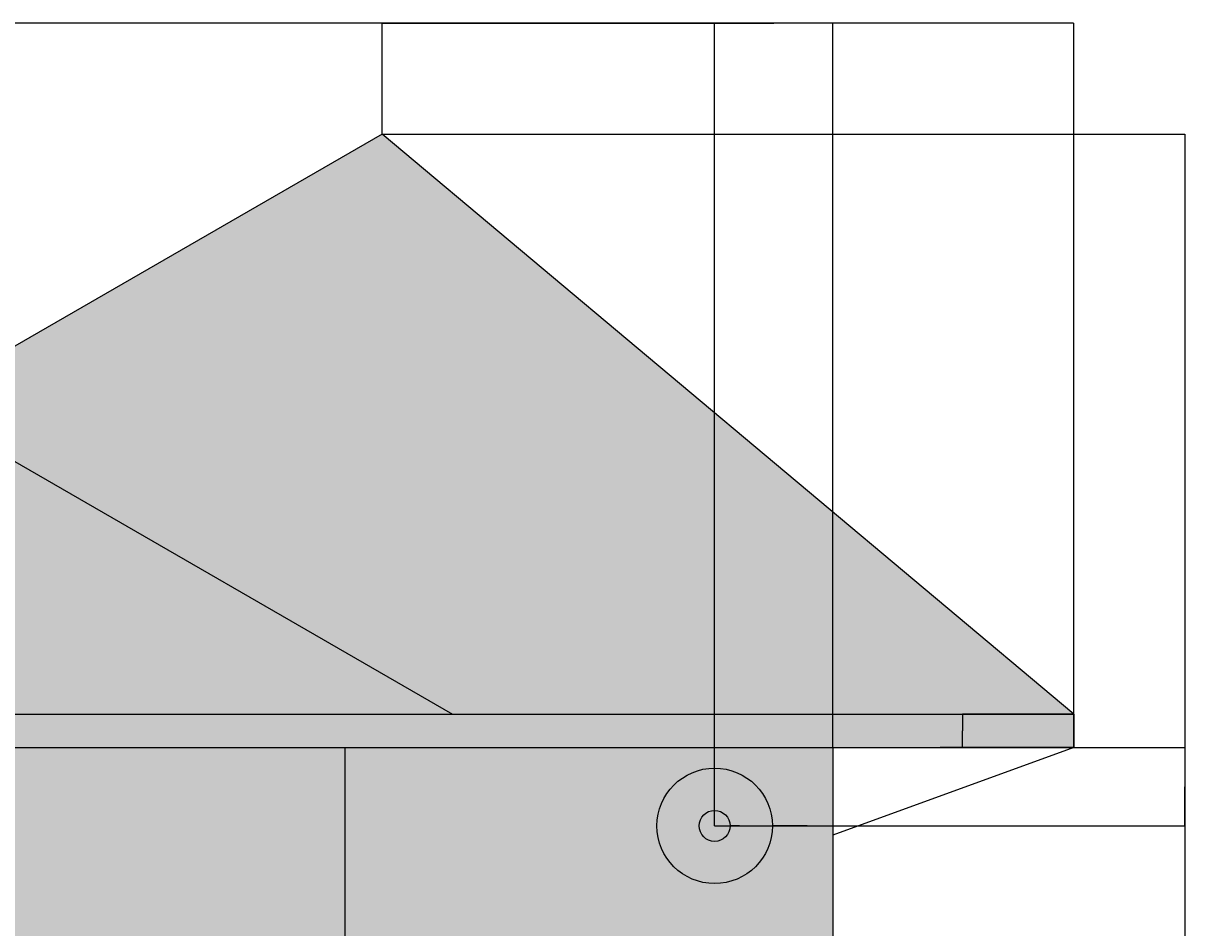
# Model space of a CAD drawing. Units: millimetres. Extents: x 2511 to 24632, y 2213 to 12972.
# Tile 5 of 5: x 19414 to 24632, y 8906 to 12972. Entities that reach past the tile are written whole.
import ezdxf

# ---------------------------------------------------------------- set-up
doc = ezdxf.new("R2010")
doc.units = ezdxf.units.MM
for name, color, linetype, lineweight in [('A-ANNO-DIMS', 2, 'Continuous', 18), ('A-ELEV', 7, 'Continuous', 25), ('A-ELEV-PATT', 13, 'Continuous', 9), ('A-ROOF', 7, 'Continuous', 25), ('A-ROOF-PATT', 13, 'Continuous', 13)]:
    doc.layers.add(name, color=color, linetype=linetype, lineweight=lineweight)
doc.styles.get("Standard").update_dxf_attribs({"font": 'arial.ttf'})
doc.dimstyles.get("Standard").update_dxf_attribs({"dimtxt": 0.18, "dimasz": 0.18, "dimexe": 0.18, "dimexo": 0.0625, "dimgap": 0.09, "dimtad": 0, "dimtih": 1, "dimtoh": 1, "dimdec": 4, "dimzin": 0, "dimdsep": 46, "dimtxsty": 'Standard', "dimcen": 0.09, "dimadec": 0, "dimazin": 0, "dimtfac": 1, "dimtdec": 4, "dimtofl": 0, "dimtmove": 0, "dimatfit": 3, "dimfxl": 1, "dimtolj": 1, "dimtzin": 0, "dimarcsym": 0})

# ---------------------------------------------------------------- blocks, each defined once
blk = doc.blocks.new('*D64')
at = {"layer": 'A-ANNO-DIMS', "color": 0, "lineweight": -2, "transparency": 16777216}
for p, q in [((14162.809797, 9866.279030000002), (14162.809797, 12971.685584)), ((14162.989797, 12971.505584), (19147.45133178854, 12971.505584)), ((24132.629797, 12971.505584), (19148.16826221146, 12971.505584)), ((24132.809797, 9716.27903), (24132.809797, 12971.685584))]:
    blk.add_line(p, q, dxfattribs=at)
at = {"layer": 'A-ANNO-DIMS', "color": 0, "transparency": 16777216}
for points in [[(14162.989797, 12971.535584), (14162.989797, 12971.475584), (14162.809797, 12971.505584)], [(24132.629797, 12971.535584), (24132.629797, 12971.475584), (24132.809797, 12971.505584)]]:
    blk.add_solid(points, dxfattribs=at)
at = {"layer": 'Defpoints', "color": 0, "transparency": 16777216}
for p in [(14162.809797, 12971.505584), (14162.809797, 9866.21653), (24132.809797, 9716.21653)]:
    blk.add_point(p, dxfattribs=at)
at = {"layer": 'A-ANNO-DIMS', "color": 0, "transparency": 16777216, "insert": (19147.809797, 12971.505584), "char_height": 0.18, "attachment_point": 5}
blk.add_mtext('\\A1;9970', dxfattribs=at)
blk = doc.blocks.new('*D65')
at = {"layer": 'A-ANNO-DIMS', "color": 0, "lineweight": -2, "transparency": 16777216}
for p, q in [((21026.52001400001, 12472.75558400001), (24631.73979700003, 12472.75558400001)), ((24631.55979700003, 12472.575584), (24631.55979700003, 7739.667960137794)), ((24631.55979700003, 3006.396530000001), (24631.55979700003, 7739.304153862214)), ((23938.87229700001, 3006.216530000001), (24631.73979700003, 3006.216530000001))]:
    blk.add_line(p, q, dxfattribs=at)
at = {"layer": 'A-ANNO-DIMS', "color": 0, "transparency": 16777216}
for points in [[(24631.52979700003, 12472.575584), (24631.58979700003, 12472.575584), (24631.55979700003, 12472.75558400001)], [(24631.52979700003, 3006.396530000001), (24631.58979700003, 3006.396530000001), (24631.55979700003, 3006.216530000001)]]:
    blk.add_solid(points, dxfattribs=at)
at = {"layer": 'Defpoints', "color": 0, "transparency": 16777216}
for p in [(21026.45751400001, 12472.75558400001), (24631.55979700003, 12472.75558400001), (23938.80979700001, 3006.216530000001)]:
    blk.add_point(p, dxfattribs=at)
at = {"layer": 'A-ANNO-DIMS', "color": 0, "transparency": 16777216, "insert": (24631.55979700002, 7739.486056999995), "char_height": 0.18, "attachment_point": 5}
blk.add_mtext('\\A1;9467', dxfattribs=at)
blk = doc.blocks.new('*D83')
at = {"layer": 'A-ANNO-DIMS', "color": 0, "lineweight": -2, "transparency": 16777216}
for p, q in [((24132.74729700001, 9866.216530000003), (23633.87979700002, 9866.216530000003)), ((23634.05979700002, 9866.036530000005), (23634.05979700002, 9791.398433137792)), ((23634.05979700002, 9716.396530000004), (23634.05979700002, 9791.034626862214)), ((24132.74729700001, 9716.216530000003), (23633.87979700002, 9716.216530000003))]:
    blk.add_line(p, q, dxfattribs=at)
at = {"layer": 'A-ANNO-DIMS', "color": 0, "transparency": 16777216}
for points in [[(23634.02979700002, 9866.036530000005), (23634.08979700002, 9866.036530000005), (23634.05979700002, 9866.216530000003)], [(23634.02979700002, 9716.396530000004), (23634.08979700002, 9716.396530000004), (23634.05979700002, 9716.216530000003)]]:
    blk.add_solid(points, dxfattribs=at)
at = {"layer": 'Defpoints', "color": 0, "transparency": 16777216}
for p in [(23634.05979700002, 9866.216530000003), (24132.80979700001, 9866.216530000003), (24132.80979700001, 9716.216530000003)]:
    blk.add_point(p, dxfattribs=at)
at = {"layer": 'A-ANNO-DIMS', "color": 0, "transparency": 16777216, "insert": (23634.05979700002, 9791.216529999994), "char_height": 0.18, "attachment_point": 5}
blk.add_mtext('\\A1;150', dxfattribs=at)
blk = doc.blocks.new('*D89')
at = {"layer": 'A-ANNO-DIMS', "color": 0, "lineweight": -2, "transparency": 16777216}
for p, q in [((21026.457514, 12472.818084), (21026.457514, 12971.685584)), ((21026.637514, 12971.505584), (22579.17045631856, 12971.505584)), ((24132.629797, 12971.505584), (22580.09685468145, 12971.505584)), ((24132.809797, 9866.279030000002), (24132.809797, 12971.685584))]:
    blk.add_line(p, q, dxfattribs=at)
at = {"layer": 'A-ANNO-DIMS', "color": 0, "transparency": 16777216}
for points in [[(21026.637514, 12971.535584), (21026.637514, 12971.475584), (21026.457514, 12971.505584)], [(24132.629797, 12971.535584), (24132.629797, 12971.475584), (24132.809797, 12971.505584)]]:
    blk.add_solid(points, dxfattribs=at)
at = {"layer": 'Defpoints', "color": 0, "transparency": 16777216}
for p in [(24132.809797, 12971.505584), (21026.457514, 12472.755584), (24132.809797, 9866.21653)]:
    blk.add_point(p, dxfattribs=at)
at = {"layer": 'A-ANNO-DIMS', "color": 0, "transparency": 16777216, "insert": (22579.6336555, 12971.505584), "char_height": 0.18, "attachment_point": 5}
blk.add_mtext('\\A1;3106.4', dxfattribs=at)
blk = doc.blocks.new('*D94')
at = {"layer": 'A-ANNO-DIMS', "color": 0, "lineweight": -2, "transparency": 16777216}
for p, q in [((22519.940295, 9364.00152), (22519.940295, 12971.685584)), ((22520.120295, 12971.505584), (22785.37966104366, 12971.505584)), ((23051.426435, 12971.505584), (22786.16706895634, 12971.505584)), ((23051.606435, 9716.27903), (23051.606435, 12971.685584))]:
    blk.add_line(p, q, dxfattribs=at)
at = {"layer": 'A-ANNO-DIMS', "color": 0, "transparency": 16777216}
for points in [[(22520.120295, 12971.535584), (22520.120295, 12971.475584), (22519.940295, 12971.505584)], [(23051.426435, 12971.535584), (23051.426435, 12971.475584), (23051.606435, 12971.505584)]]:
    blk.add_solid(points, dxfattribs=at)
at = {"layer": 'Defpoints', "color": 0, "transparency": 16777216}
for p in [(23051.606435, 12971.505584), (23051.606435, 9716.21653), (22519.940295, 9363.93902)]:
    blk.add_point(p, dxfattribs=at)
at = {"layer": 'A-ANNO-DIMS', "color": 0, "transparency": 16777216, "insert": (22785.773365, 12971.505584), "char_height": 0.18, "attachment_point": 5}
blk.add_mtext('\\A1;531.7', dxfattribs=at)
blk = doc.blocks.new('*D95')
at = {"layer": 'A-ANNO-DIMS', "color": 0, "lineweight": -2, "transparency": 16777216}
for p, q in [((23051.66893500001, 9716.216530000003), (24631.73979700003, 9716.216530000003)), ((24631.55979700003, 9716.036530000003), (24631.55979700003, 9540.259739529334)), ((24631.55979700003, 9364.119020000004), (24631.55979700003, 9539.895810470673)), ((22520.00279500001, 9363.939020000003), (24631.73979700003, 9363.939020000003))]:
    blk.add_line(p, q, dxfattribs=at)
at = {"layer": 'A-ANNO-DIMS', "color": 0, "transparency": 16777216}
for points in [[(24631.52979700003, 9716.036530000003), (24631.58979700003, 9716.036530000003), (24631.55979700003, 9716.216530000003)], [(24631.52979700003, 9364.119020000004), (24631.58979700003, 9364.119020000004), (24631.55979700003, 9363.939020000003)]]:
    blk.add_solid(points, dxfattribs=at)
at = {"layer": 'Defpoints', "color": 0, "transparency": 16777216}
for p in [(23051.60643500001, 9716.216530000003), (22519.94029500001, 9363.939020000003), (24631.55979700003, 9363.939020000003)]:
    blk.add_point(p, dxfattribs=at)
at = {"layer": 'A-ANNO-DIMS', "color": 0, "transparency": 16777216, "insert": (24631.55979700003, 9540.077774999994), "char_height": 0.18, "attachment_point": 5}
blk.add_mtext('\\A1;352.3', dxfattribs=at)
blk = doc.blocks.new('*D102')
at = {"layer": 'A-ANNO-DIMS', "color": 0, "lineweight": -2, "transparency": 16777216}
for p, q in [((22519.85029499999, 9363.939020000002), (22520.03029499999, 9363.939020000003)), ((22519.940295, 9363.849020000001), (22519.940295, 9364.029020000002)), ((22935.0733398, 9363.938988000005), (22779.57844799999, 9363.93899998613))]:
    blk.add_line(p, q, dxfattribs=at)
at = {"layer": 'A-ANNO-DIMS', "color": 0, "transparency": 16777216}
blk.add_solid([(22779.57844800231, 9363.96899998613), (22779.57844799768, 9363.908999986128), (22779.39844799999, 9363.939000000002)], dxfattribs=at)
at = {"layer": 'Defpoints', "color": 0, "transparency": 16777216}
for p in [(22260.482142, 9363.939040000001), (22779.39844799999, 9363.939000000002)]:
    blk.add_point(p, dxfattribs=at)
at = {"layer": 'A-ANNO-DIMS', "color": 0, "transparency": 16777216, "insert": (22935.56514743983, 9363.938988000004), "char_height": 0.18, "attachment_point": 5}
blk.add_mtext('\\A1;∅518.9', dxfattribs=at)
blk = doc.blocks.new('*D103')
at = {"layer": 'A-ANNO-DIMS', "color": 0, "lineweight": -2, "transparency": 16777216}
for p, q in [((22519.85029500001, 9363.939020000005), (22520.03029500001, 9363.939020000003)), ((22519.940295, 9363.849020000005), (22519.940295, 9364.029020000004)), ((22631.19809499585, 9363.940589600003), (22589.65641999998, 9363.940003539403))]:
    blk.add_line(p, q, dxfattribs=at)
at = {"layer": 'A-ANNO-DIMS', "color": 0, "transparency": 16777216}
blk.add_solid([(22589.65641957675, 9363.9700035394), (22589.65642042322, 9363.910003539408), (22589.47642, 9363.940001000004)], dxfattribs=at)
at = {"layer": 'Defpoints', "color": 0, "transparency": 16777216}
for p in [(22450.40417000001, 9363.938039000002), (22589.47642, 9363.940001000004)]:
    blk.add_point(p, dxfattribs=at)
at = {"layer": 'A-ANNO-DIMS', "color": 0, "transparency": 16777216, "insert": (22631.75964342695, 9363.940589600003), "char_height": 0.18, "attachment_point": 5}
blk.add_mtext('\\A1;∅139.07', dxfattribs=at)

msp = doc.modelspace()

# ---------------------------------------------------------------- hatches: boundary and pattern name
at = {"layer": 'A-ELEV-PATT', "transparency": 33554551}
h = msp.add_hatch(color=256, dxfattribs=at)
h.dxf.hatch_style = 1
h.paths.add_polyline_path([(20858.80979657499, 6516.216530118374), (14762.80979657499, 6516.21653011837), (14762.80979657499, 3466.216530118371), (19843.80979657499, 3466.216530118371), (19843.80979657499, 5601.216530118371), (20718.80979657499, 5601.216530118371), (20718.80979657499, 3466.216530118371), (20858.80979657499, 3466.216530118371)])
h.paths.add_polyline_path([(16969.80319715291, 5601.216530118371), (16969.80319715291, 4381.21653011837), (15441.81503455806, 4381.21653011837), (15441.81503455806, 5601.216530118371)], flags=16)
h.paths.add_polyline_path([(16919.80319715291, 5551.21653011837), (16919.80319715291, 4431.21653011837), (15491.81503455806, 4431.21653011837), (15491.81503455806, 5551.21653011837)], flags=0)
h.paths.add_polyline_path([(17877.81880597513, 5601.216530118371), (19413.9915447958, 5601.216530118371), (19413.9915447958, 4381.21653011837), (17886.00338220095, 4381.21653011837), (17877.81880597513, 4381.21653011837)], flags=16)
h.paths.add_polyline_path([(17936.00338220095, 5551.21653011837), (19363.9915447958, 5551.21653011837), (19363.9915447958, 4431.21653011837), (17936.00338220095, 4431.21653011837)], flags=0)
h.paths.add_polyline_path([(20858.80979657499, 9716.216530118376), (14762.80979657499, 9716.21653011837), (14762.80979657499, 6666.21653011837), (19522.169078361, 6666.21653011837), (19522.169078361, 7733.216530118371), (20858.80979657499, 7733.216530118371)])
h.paths.add_polyline_path([(16969.80319715291, 8801.21653011837), (16969.80319715291, 7581.216530118371), (15441.81503455806, 7581.216530118371), (15441.81503455806, 8801.21653011837)], flags=16)
h.paths.add_polyline_path([(16919.80319715291, 8751.216530118369), (16919.80319715291, 7631.216530118371), (15491.81503455806, 7631.216530118371), (15491.81503455806, 8751.216530118369)], flags=0)
h.paths.add_polyline_path([(17877.81880597514, 8801.21653011837), (19413.9915447958, 8801.21653011837), (19413.9915447958, 7581.216530118371), (17886.00338220095, 7581.216530118371), (17877.81880597513, 7581.216530118371)], flags=16)
h.paths.add_polyline_path([(17936.00338220095, 8751.216530118369), (19363.9915447958, 8751.216530118369), (19363.9915447958, 7631.216530118371), (17936.00338220095, 7631.216530118371)], flags=0)
h.paths.add_polyline_path([(23051.60643531334, 9716.216530118376), (20858.80979657499, 9716.21653011837), (20858.80979657499, 7733.216530118371), (23051.60643531334, 7733.216530118371)])
h.paths.add_polyline_path([(23051.60643531335, 6516.216530118374), (20858.80979657499, 6516.216530118374), (20858.80979657499, 3516.21653011837), (23051.60643531335, 3516.21653011837)])
at = {"layer": 'A-ROOF-PATT'}
h = msp.add_hatch(dxfattribs=at)
h.set_pattern_fill('ANGLE', color=256, scale=15)
h.set_pattern_definition([(0, (11792.595132882, -12295.09862892571), (0, 104.775), [76.2, -28.575]), (90, (11792.595132882, -12295.09862892571), (-104.775, 6.4e-15), [76.2, -28.575])])
h.paths.add_polyline_path([(17752.26282908254, 11938.58820468012), (14162.80979657499, 9866.216530118376), (14762.80979657499, 9866.216530118376), (15511.62610781541, 9866.216530118376), (17061.36801812783, 10760.96043921169), (18611.10992844025, 9866.216530118376), (21341.71586159009, 9866.21653011837)])
h.paths.add_polyline_path([(21026.45751448832, 12472.755584324), (18926.75765114087, 11260.49330300292), (21341.71586159008, 9866.21653011837), (23532.80979657499, 9866.21653011837), (24132.80979657499, 9866.21653011837)])
h.paths.add_polyline_path([(17061.36801812783, 10760.96043921169), (15511.62610781541, 9866.216530118376), (18611.10992844025, 9866.21653011837)], flags=17)
at = {"layer": 'A-ROOF-PATT', "transparency": 33554551}
h = msp.add_hatch(color=256, dxfattribs=at)
h.dxf.hatch_style = 1
h.paths.add_polyline_path([(24132.80979657499, 9866.21653011837), (23532.80979657499, 9866.21653011837), (14762.80979657499, 9866.216530118376), (14162.80979657499, 9866.216530118376), (14162.80979657499, 9716.21653011837), (14762.80979657499, 9716.21653011837), (23532.80979657499, 9716.216530118376), (24132.80979657499, 9716.216530118376)])

# ---------------------------------------------------------------- linework, layer by layer
at = {"layer": 'A-ELEV'}
for p, q in [((20858.80979657499, 9716.21653011837), (20858.80979657499, 7733.216530118371)), ((23051.60643531334, 9716.216530118376), (23051.60643531334, 7733.216530118371))]:
    msp.add_line(p, q, dxfattribs=at)
for radius in [259.45815263642, 69.53612460638396]:
    msp.add_circle((22519.94029529997, 9363.939019813582), radius, dxfattribs=at)
at = {"layer": 'A-ROOF'}
for p, q in [((21026.45751448832, 12472.755584324), (18926.75765114087, 11260.49330300292)), ((24132.80979657499, 9866.21653011837), (21026.45751448832, 12472.755584324)), ((17752.26282908254, 11938.58820468012), (21341.71586159009, 9866.21653011837)), ((14762.80979657499, 9866.216530118376), (23532.80979657499, 9866.21653011837)), ((23532.80979657499, 9866.21653011837), (24132.80979657499, 9866.21653011837)), ((24132.80979657499, 9866.21653011837), (24132.80979657499, 9716.216530118376)), ((14762.80979657499, 9716.21653011837), (23532.80979657499, 9716.216530118376)), ((24132.80979657499, 9716.216530118376), (23051.60643531334, 9322.690689430565)), ((24132.80979657499, 9716.216530118376), (23532.80979657499, 9716.216530118376))]:
    msp.add_line(p, q, dxfattribs=at)

# ---------------------------------------------------------------- dimensions: what is measured, and where the dimension line sits
at = {"layer": 'A-ANNO-DIMS'}
for base, p1, p2, override, picture, middle in [((14162.809797, 12971.505584), (24132.809797, 9716.21653), (14162.809797, 9866.21653), {"dimdec": 0, "dimlfac": 1, "dimrnd": 0, "dimzin": 0, "dimdsep": 46, "dimlunit": 2}, '*D64', (19147.809797, 12971.505584)), ((24132.809797, 12971.505584), (21026.457514, 12472.755584), (24132.809797, 9866.21653), {"dimdec": 1, "dimlfac": 1, "dimrnd": 0, "dimzin": 0, "dimdsep": 46, "dimlunit": 2}, '*D89', (22579.6336555, 12971.505584)), ((23051.606435, 12971.505584), (22519.940295, 9363.93902), (23051.606435, 9716.21653), {"dimdec": 1, "dimlfac": 1, "dimrnd": 0, "dimzin": 0, "dimdsep": 46, "dimlunit": 2}, '*D94', (22785.773365, 12971.505584))]:
    dim = msp.add_linear_dim(base=base, p1=p1, p2=p2, dimstyle='Standard', override=override, dxfattribs=at)
    dim.commit()
    dim.dimension.update_dxf_attribs({"geometry": picture, "text_midpoint": middle})
for base, p1, p2, override, picture, middle in [((24631.55979700003, 12472.75558400001), (23938.809797, 3006.21653), (21026.457514, 12472.755584), {"dimdec": 0, "dimlfac": 1, "dimrnd": 0, "dimzin": 0, "dimdsep": 46, "dimlunit": 2}, '*D65', (24631.55979700002, 7739.486056999995)), ((23634.05979700002, 9866.216530000003), (24132.809797, 9716.21653), (24132.809797, 9866.21653), {"dimdec": 0, "dimlfac": 1, "dimrnd": 0, "dimzin": 0, "dimdsep": 46, "dimlunit": 2}, '*D83', (23634.05979700002, 9791.216529999994)), ((24631.55979700003, 9363.939020000003), (23051.606435, 9716.21653), (22519.940295, 9363.93902), {"dimdec": 1, "dimlfac": 1, "dimrnd": 0, "dimzin": 0, "dimdsep": 46, "dimlunit": 2}, '*D95', (24631.55979700003, 9540.077774999994))]:
    dim = msp.add_linear_dim(base=base, p1=p1, p2=p2, angle=90, dimstyle='Standard', override=override, dxfattribs=at)
    dim.commit()
    dim.dimension.update_dxf_attribs({"geometry": picture, "text_midpoint": middle})
for p1, p2, override, picture, middle in [((22260.482142, 9363.939040000001), (22779.39844799999, 9363.939000000002), {"dimdec": 1, "dimlfac": 1, "dimrnd": 0, "dimzin": 0, "dimdsep": 46, "dimlunit": 2}, '*D102', (22935.0733398, 9363.938988000005)), ((22450.40417000001, 9363.938039000002), (22589.47642, 9363.940001000004), {"dimdec": 2, "dimlfac": 1, "dimrnd": 0, "dimzin": 0, "dimdsep": 46, "dimlunit": 2}, '*D103', (22631.19809499585, 9363.940589600003))]:
    dim = msp.add_diameter_dim_2p(p1=p1, p2=p2, dimstyle='Standard', override=override, dxfattribs=at)
    dim.commit()
    dim.dimension.update_dxf_attribs({"geometry": picture, "text_midpoint": middle, "dimtype": 163})

doc.saveas('drawing.dxf')
